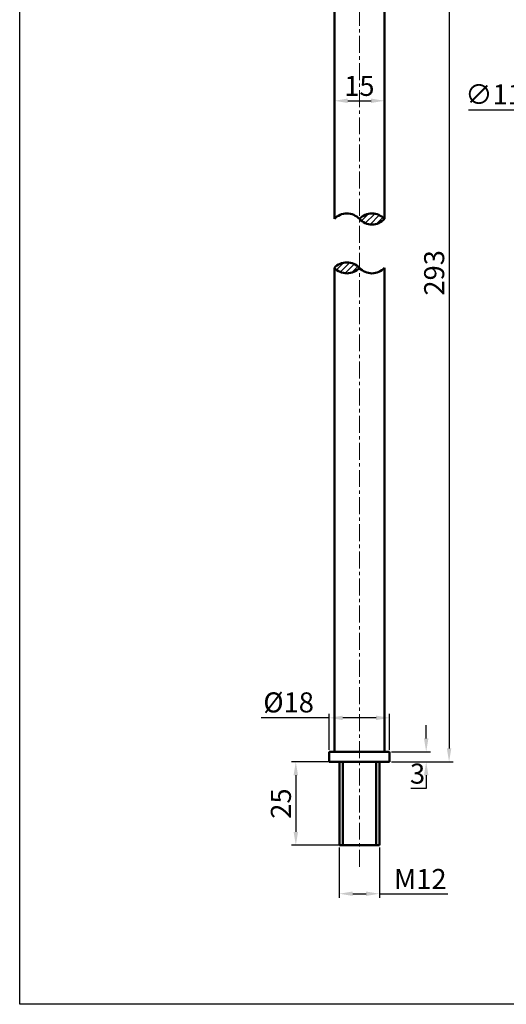
# Model space of a CAD drawing. Units: millimetres. Extents: x -65 to 576, y -103 to 374.
# Tile 1 of 4: x -65 to 81, y -103 to 192. Entities that reach past the tile are written whole.
import ezdxf

# ---------------------------------------------------------------- set-up
doc = ezdxf.new("R2010")
doc.units = ezdxf.units.MM
doc.header["$LTSCALE"] = 0.4
doc.linetypes.add('CENTER', pattern=[50.8, 31.75, -6.35, 6.35, -6.35])
for name, color, linetype, lineweight in [('M-CNTR', 4, 'CENTER', 18), ('M-DIMS', 2, 'Continuous', 25), ('M-HATC', 8, 'Continuous', 18), ('M-OUTL', 7, 'Continuous', 50), ('M-TTLB', 7, 'Continuous', 25)]:
    doc.layers.add(name, color=color, linetype=linetype, lineweight=lineweight)
doc.styles.get("Standard").update_dxf_attribs({"font": 'arial.ttf'})
doc.dimstyles.new('ISO-25', dxfattribs={"dimtxt": 6, "dimasz": 4, "dimexe": 1.25, "dimexo": 0.625, "dimtad": 1, "dimtoh": 1, "dimtxsty": 'Standard', "dimcen": 2.5, "dimadec": 0, "dimazin": 0, "dimtfac": 1, "dimtofl": 0, "dimtmove": 0, "dimatfit": 3, "dimfxl": 1, "dimarcsym": 0})

# ---------------------------------------------------------------- blocks, each defined once
blk = doc.blocks.new('*D11')
at = {"layer": 'Defpoints', "color": 0, "ltscale": 0.4, "transparency": 16777216}
for p in [(29.59, 187.77), (44.59, 187.77), (44.59, 167.33)]:
    blk.add_point(p, dxfattribs=at)
at = {"layer": 'M-DIMS', "color": 0, "lineweight": -2, "ltscale": 0.4, "transparency": 16777216}
for p, q in [((29.59, 187.14), (29.59, 166.08)), ((44.59, 187.14), (44.59, 166.08)), ((33.59, 167.33), (40.59, 167.33))]:
    blk.add_line(p, q, dxfattribs=at)
at = {"layer": 'M-DIMS', "color": 0, "ltscale": 0.4, "transparency": 16777216}
for points in [[(33.59, 168), (33.59, 166.67), (29.59, 167.33)], [(40.59, 168), (40.59, 166.67), (44.59, 167.33)]]:
    blk.add_solid(points, dxfattribs=at)
at = {"layer": 'M-DIMS', "color": 0, "ltscale": 0.4, "transparency": 16777216, "insert": (37.09, 171.02), "char_height": 6, "attachment_point": 5}
blk.add_mtext('15', dxfattribs=at)
blk = doc.blocks.new('*D12')
at = {"layer": 'Defpoints', "color": 0, "ltscale": 0.4, "transparency": 16777216}
for p in [(44.59, 262.28), (46.09, -30.72), (63.96, -30.72)]:
    blk.add_point(p, dxfattribs=at)
at = {"layer": 'M-DIMS', "color": 0, "lineweight": -2, "ltscale": 0.4, "transparency": 16777216}
for p, q in [((45.22, 262.28), (65.21, 262.28)), ((63.96, 258.28), (63.96, -26.72)), ((46.72, -30.72), (65.21, -30.72))]:
    blk.add_line(p, q, dxfattribs=at)
at = {"layer": 'M-DIMS', "color": 0, "ltscale": 0.4, "transparency": 16777216}
for points in [[(63.29, 258.28), (64.63, 258.28), (63.96, 262.28)], [(63.29, -26.72), (64.63, -26.72), (63.96, -30.72)]]:
    blk.add_solid(points, dxfattribs=at)
at = {"layer": 'M-DIMS', "color": 0, "ltscale": 0.4, "transparency": 16777216, "insert": (60.27, 115.78), "char_height": 6, "attachment_point": 5, "rotation": 90}
blk.add_mtext('293', dxfattribs=at)
blk = doc.blocks.new('*D13')
at = {"layer": 'Defpoints', "color": 0, "ltscale": 0.4, "transparency": 16777216}
for p in [(31.09, -55.72), (43.09, -55.72), (43.09, -70.23)]:
    blk.add_point(p, dxfattribs=at)
at = {"layer": 'M-DIMS', "color": 0, "lineweight": -2, "ltscale": 0.4, "transparency": 16777216}
for p, q in [((31.09, -56.34), (31.09, -71.48)), ((43.09, -56.34), (43.09, -71.48)), ((35.09, -70.23), (39.09, -70.23)), ((43.09, -70.23), (63.59, -70.23))]:
    blk.add_line(p, q, dxfattribs=at)
at = {"layer": 'M-DIMS', "color": 0, "ltscale": 0.4, "transparency": 16777216}
for points in [[(35.09, -69.57), (35.09, -70.9), (31.09, -70.23)], [(39.09, -69.57), (39.09, -70.9), (43.09, -70.23)]]:
    blk.add_solid(points, dxfattribs=at)
at = {"layer": 'M-DIMS', "color": 0, "ltscale": 0.4, "transparency": 16777216, "insert": (55.34, -66.6), "char_height": 6, "attachment_point": 5}
blk.add_mtext('M12', dxfattribs=at)
blk = doc.blocks.new('*D14')
at = {"layer": 'Defpoints', "color": 0, "ltscale": 0.4, "transparency": 16777216}
for p in [(46.09, -27.72), (46.09, -30.72), (57.1, -30.72)]:
    blk.add_point(p, dxfattribs=at)
at = {"layer": 'M-DIMS', "color": 0, "lineweight": -2, "ltscale": 0.4, "transparency": 16777216}
for p, q in [((57.1, -23.72), (57.1, -19.72)), ((46.72, -27.72), (58.35, -27.72)), ((46.72, -30.72), (58.35, -30.72)), ((57.1, -34.72), (57.1, -38.72)), ((57.1, -38.72), (52.55, -38.72))]:
    blk.add_line(p, q, dxfattribs=at)
at = {"layer": 'M-DIMS', "color": 0, "ltscale": 0.4, "transparency": 16777216}
for points in [[(56.43, -23.72), (57.77, -23.72), (57.1, -27.72)], [(56.43, -34.72), (57.77, -34.72), (57.1, -30.72)]]:
    blk.add_solid(points, dxfattribs=at)
at = {"layer": 'M-DIMS', "color": 0, "ltscale": 0.4, "transparency": 16777216, "insert": (54.51, -35.03), "char_height": 6, "attachment_point": 5}
blk.add_mtext('3', dxfattribs=at)
blk = doc.blocks.new('*D15')
at = {"layer": 'Defpoints', "color": 0, "ltscale": 0.4, "transparency": 16777216}
for p in [(46.09, -17.54), (28.09, -27.72), (46.09, -27.72)]:
    blk.add_point(p, dxfattribs=at)
at = {"layer": 'M-DIMS', "color": 0, "lineweight": -2, "ltscale": 0.4, "transparency": 16777216}
for p, q in [((28.09, -17.54), (7.71, -17.54)), ((28.09, -27.09), (28.09, -16.29)), ((42.09, -17.54), (32.09, -17.54)), ((46.09, -27.09), (46.09, -16.29))]:
    blk.add_line(p, q, dxfattribs=at)
at = {"layer": 'M-DIMS', "color": 0, "ltscale": 0.4, "transparency": 16777216}
for points in [[(32.09, -16.88), (32.09, -18.21), (28.09, -17.54)], [(42.09, -16.88), (42.09, -18.21), (46.09, -17.54)]]:
    blk.add_solid(points, dxfattribs=at)
at = {"layer": 'M-DIMS', "color": 0, "ltscale": 0.4, "transparency": 16777216, "insert": (15.9, -13.69), "char_height": 6, "attachment_point": 5}
blk.add_mtext('%%C18', dxfattribs=at)
blk = doc.blocks.new('*D16')
at = {"layer": 'Defpoints', "color": 0, "ltscale": 0.4, "transparency": 16777216}
for p in [(37.09, -30.72), (18.06, -55.72), (37.09, -55.72)]:
    blk.add_point(p, dxfattribs=at)
at = {"layer": 'M-DIMS', "color": 0, "lineweight": -2, "ltscale": 0.4, "transparency": 16777216}
for p, q in [((36.47, -30.72), (16.81, -30.72)), ((18.06, -34.72), (18.06, -51.72)), ((36.47, -55.72), (16.81, -55.72))]:
    blk.add_line(p, q, dxfattribs=at)
at = {"layer": 'M-DIMS', "color": 0, "ltscale": 0.4, "transparency": 16777216}
for points in [[(17.39, -34.72), (18.73, -34.72), (18.06, -30.72)], [(17.39, -51.72), (18.73, -51.72), (18.06, -55.72)]]:
    blk.add_solid(points, dxfattribs=at)
at = {"layer": 'M-DIMS', "color": 0, "ltscale": 0.4, "transparency": 16777216, "insert": (14.37, -43.22), "char_height": 6, "attachment_point": 5, "rotation": 90}
blk.add_mtext('25', dxfattribs=at)
blk = doc.blocks.new('*D56')
at = {"layer": 'Defpoints', "color": 0, "ltscale": 0.4, "transparency": 16777216}
for p in [(119.8, 147.5), (218.49, 90.42)]:
    blk.add_point(p, dxfattribs=at)
at = {"layer": 'M-DIMS', "color": 0, "lineweight": -2, "ltscale": 0.4, "transparency": 16777216}
for p, q in [((69.82, 164.62), (90.2, 164.62)), ((90.2, 164.62), (116.34, 149.5)), ((169.15, 116.46), (169.15, 121.46)), ((166.65, 118.96), (171.65, 118.96))]:
    blk.add_line(p, q, dxfattribs=at)
at = {"layer": 'M-DIMS', "color": 0, "ltscale": 0.4, "transparency": 16777216}
blk.add_solid([(116.68, 150.08), (116.01, 148.92), (119.8, 147.5)], dxfattribs=at)
at = {"layer": 'M-DIMS', "color": 0, "ltscale": 0.4, "transparency": 16777216, "insert": (79.7, 168.48), "char_height": 6, "attachment_point": 5}
blk.add_mtext('∅114', dxfattribs=at)

msp = doc.modelspace()

# ---------------------------------------------------------------- hatches: boundary and pattern name
at = {"layer": 'M-HATC', "ltscale": 0.4}
h = msp.add_hatch(dxfattribs=at)
h.set_pattern_fill('ANSI31', color=256, scale=0.4)
h.set_pattern_definition([(45, (-414.4572, 41.9653), (-0.8980256, 0.8980256), [])])
h.paths.add_polyline_path([(44.594, 131.923, 0.4399217), (37.094, 131.923, 0.4399217)])
h.paths.add_polyline_path([(29.594, 117.281, 0.4399217), (37.094, 117.281, 0.4399217)])

# ---------------------------------------------------------------- linework, layer by layer
at = {"layer": 'M-CNTR', "ltscale": 0.4}
msp.add_line((37.094, -62.16), (37.094, 286.009), dxfattribs=at)
at = {"layer": 'M-OUTL', "ltscale": 0.4}
for p, q in [((29.594, 262.281), (29.594, 131.923)), ((44.594, 262.281), (44.594, 131.923)), ((29.594, 117.281), (29.594, -27.719)), ((44.594, 117.281), (44.594, -27.719)), ((44.594, -27.719), (28.094, -27.719)), ((28.094, -27.719), (28.094, -30.719)), ((46.094, -27.719), (44.594, -27.719)), ((46.094, -30.719), (46.094, -27.719)), ((28.094, -30.719), (46.094, -30.719)), ((31.094, -55.719), (31.094, -30.719)), ((32.094, -55.719), (32.094, -30.719)), ((42.094, -30.719), (42.094, -55.719)), ((43.094, -30.719), (43.094, -55.719)), ((43.094, -55.719), (31.094, -55.719))]:
    msp.add_line(p, q, dxfattribs=at)
for centre, start, end in [((33.344, 128.485), 42.50853, 137.49147), ((40.844, 128.485), 42.50853, 137.49147), ((40.844, 135.36), 222.50853, 317.49147), ((33.344, 113.843), 42.50853, 137.49147), ((33.344, 120.718), 222.50853, 317.49147), ((40.844, 120.718), 222.50853, 317.49147)]:
    msp.add_arc(centre, 5.087, start, end, dxfattribs=at)
at = {"layer": 'M-TTLB', "ltscale": 0.4}
msp.add_lwpolyline([(-64.629, 373.834), (576.345, 373.834), (576.345, -103.363), (-64.629, -103.363)], close=True, dxfattribs=at)

# ---------------------------------------------------------------- dimensions: what is measured, and where the dimension line sits
at = {"layer": 'M-DIMS', "ltscale": 0.4}
for base, p1, p2, picture, middle in [((63.961, -30.719), (44.594, 262.281), (46.094, -30.719), '*D12', (60.271, 115.781)), ((57.101, -30.719), (46.094, -27.719), (46.094, -30.719), '*D14', (54.511, -35.029)), ((18.06, -55.719), (37.094, -30.719), (37.094, -55.719), '*D16', (14.372, -43.219))]:
    dim = msp.add_linear_dim(base=base, p1=p1, p2=p2, angle=90, dimstyle='ISO-25', override={"dimclrd": 0, "dimclre": 0, "dimclrt": 0}, dxfattribs=at)
    dim.commit()
    dim.dimension.update_dxf_attribs({"geometry": picture, "text_midpoint": middle})
dim = msp.add_linear_dim(base=(44.594, 167.334), p1=(29.594, 187.768), p2=(44.594, 187.768), dimstyle='ISO-25', override={"dimclrd": 0, "dimclre": 0, "dimclrt": 0}, dxfattribs=at)
dim.commit()
dim.dimension.update_dxf_attribs({"geometry": '*D11', "text_midpoint": (37.094, 167.334), "dimtype": 160})
dim = msp.add_diameter_dim_2p(p1=(218.486, 90.418), p2=(119.805, 147.497), dimstyle='ISO-25', override={"dimdec": 0, "dimlfac": 1, "dimrnd": 0, "dimzin": 0, "dimdsep": 46, "dimlunit": 2}, dxfattribs=at)
dim.commit()
dim.dimension.update_dxf_attribs({"geometry": '*D56', "text_midpoint": (79.696, 164.621), "dimtype": 163})
dim = msp.add_linear_dim(base=(46.094, -17.544), p1=(28.094, -27.719), p2=(46.094, -27.719), text='%%C<>', dimstyle='ISO-25', override={"dimclrd": 0, "dimclre": 0, "dimclrt": 0}, dxfattribs=at)
dim.commit()
dim.dimension.update_dxf_attribs({"geometry": '*D15', "text_midpoint": (15.901, -17.544), "dimtype": 160})
dim = msp.add_linear_dim(base=(43.094, -70.233), p1=(31.094, -55.719), p2=(43.094, -55.719), text='M<>', dimstyle='ISO-25', override={"dimclrd": 0, "dimclre": 0, "dimclrt": 0}, dxfattribs=at)
dim.commit()
dim.dimension.update_dxf_attribs({"geometry": '*D13', "text_midpoint": (55.339, -66.595)})

doc.saveas('drawing.dxf')
